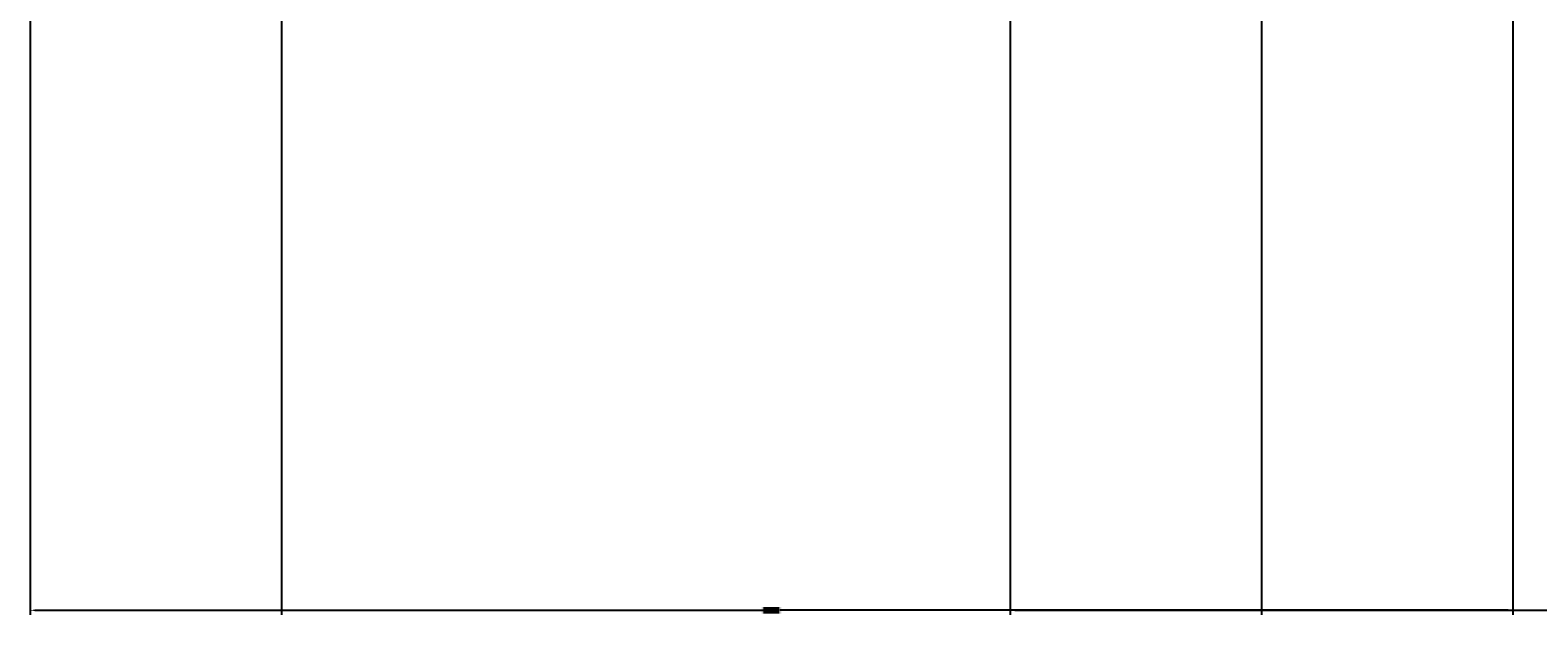
# Model space of a CAD drawing. Units: inches. Extents: x -128 to 854, y -395 to 398.
# Tile 3 of 61: x -76 to -16, y -382 to -359. Entities that reach past the tile are written whole.
import ezdxf

# ---------------------------------------------------------------- set-up
doc = ezdxf.new("R2010")
doc.units = ezdxf.units.IN
doc.header["$MEASUREMENT"] = 0
doc.layers.add('A-ANNO-DIMS', color=2, linetype='Continuous', lineweight=18)
doc.styles.get("Standard").update_dxf_attribs({"font": 'arial.ttf'})
doc.dimstyles.get("Standard").update_dxf_attribs({"dimtxt": 0.18, "dimasz": 0.18, "dimexe": 0.18, "dimexo": 0.0625, "dimgap": 0.09, "dimtad": 0, "dimtih": 1, "dimtoh": 1, "dimdec": 1, "dimzin": 0, "dimdsep": 46, "dimlunit": 4, "dimtxsty": 'Standard', "dimcen": 0.09, "dimclrd": 1, "dimclre": 2, "dimclrt": 6, "dimadec": 0, "dimazin": 0, "dimtfac": 1, "dimtdec": 1, "dimtofl": 0, "dimtmove": 0, "dimatfit": 3, "dimfxl": 1, "dimtfill": 2, "dimtfillclr": 3, "dimtolj": 1, "dimtzin": 0, "dimarcsym": 0})

# ---------------------------------------------------------------- blocks, each defined once
blk = doc.blocks.new('*D122')
at = {"layer": 'A-ANNO-DIMS', "color": 2, "lineweight": -2, "transparency": 16777216}
for p, q in [((-76.161, -358.082), (-76.161, -381.899)), ((-17.161, -358.082), (-17.161, -381.899))]:
    blk.add_line(p, q, dxfattribs=at)
at = {"layer": 'A-ANNO-DIMS', "color": 1, "lineweight": -2, "transparency": 16777216}
for p, q in [((-75.981, -381.719), (-47.064, -381.719)), ((-17.341, -381.719), (-46.258, -381.719))]:
    blk.add_line(p, q, dxfattribs=at)
at = {"layer": 'A-ANNO-DIMS', "color": 1, "transparency": 16777216}
for points in [[(-75.981, -381.689), (-75.981, -381.749), (-76.161, -381.719)], [(-17.341, -381.689), (-17.341, -381.749), (-17.161, -381.719)]]:
    blk.add_solid(points, dxfattribs=at)
at = {"layer": 'Defpoints', "color": 0, "transparency": 16777216}
for p in [(-76.161, -358.019), (-17.161, -358.019), (-17.161, -381.719)]:
    blk.add_point(p, dxfattribs=at)
at = {"layer": 'A-ANNO-DIMS', "color": 6, "transparency": 16777216, "insert": (-46.661, -381.719), "char_height": 0.18, "attachment_point": 5, "bg_fill": 1, "box_fill_scale": 1.25, "bg_fill_color": 3, "bg_fill_transparency": 0}
blk.add_mtext('\\A1;4\'-11"', dxfattribs=at)
blk = doc.blocks.new('*D123')
at = {"layer": 'A-ANNO-DIMS', "color": 2, "lineweight": -2, "transparency": 16777216}
for p, q in [((-17.161, -358.082), (-17.161, -381.899)), ((121.839, -358.082), (121.839, -381.899))]:
    blk.add_line(p, q, dxfattribs=at)
at = {"layer": 'A-ANNO-DIMS', "color": 1, "lineweight": -2, "transparency": 16777216}
for p, q in [((-16.981, -381.719), (51.948, -381.719)), ((121.659, -381.719), (52.73, -381.719))]:
    blk.add_line(p, q, dxfattribs=at)
at = {"layer": 'A-ANNO-DIMS', "color": 1, "transparency": 16777216}
for points in [[(-16.981, -381.689), (-16.981, -381.749), (-17.161, -381.719)], [(121.659, -381.689), (121.659, -381.749), (121.839, -381.719)]]:
    blk.add_solid(points, dxfattribs=at)
at = {"layer": 'Defpoints', "color": 0, "transparency": 16777216}
for p in [(-17.161, -358.019), (121.839, -358.019), (121.839, -381.719)]:
    blk.add_point(p, dxfattribs=at)
at = {"layer": 'A-ANNO-DIMS', "color": 6, "transparency": 16777216, "insert": (52.339, -381.719), "char_height": 0.18, "attachment_point": 5, "bg_fill": 1, "box_fill_scale": 1.25, "bg_fill_color": 3, "bg_fill_transparency": 0}
blk.add_mtext('\\A1;11\'-7"', dxfattribs=at)
blk = doc.blocks.new('*D125')
at = {"layer": 'A-ANNO-DIMS', "color": 2, "lineweight": -2, "transparency": 16777216}
for p, q in [((-37.161, -298.082), (-37.161, -381.899)), ((22.811, -298.082), (22.811, -381.899))]:
    blk.add_line(p, q, dxfattribs=at)
at = {"layer": 'A-ANNO-DIMS', "color": 1, "lineweight": -2, "transparency": 16777216}
for p, q in [((-36.981, -381.719), (-7.504, -381.719)), ((22.631, -381.719), (-6.846, -381.719))]:
    blk.add_line(p, q, dxfattribs=at)
at = {"layer": 'A-ANNO-DIMS', "color": 1, "transparency": 16777216}
for points in [[(-36.981, -381.689), (-36.981, -381.749), (-37.161, -381.719)], [(22.631, -381.689), (22.631, -381.749), (22.811, -381.719)]]:
    blk.add_solid(points, dxfattribs=at)
at = {"layer": 'Defpoints', "color": 0, "transparency": 16777216}
for p in [(-37.161, -298.019), (22.811, -298.019), (22.811, -381.719)]:
    blk.add_point(p, dxfattribs=at)
at = {"layer": 'A-ANNO-DIMS', "color": 6, "transparency": 16777216, "insert": (-7.175, -381.719), "char_height": 0.18, "attachment_point": 5, "bg_fill": 1, "box_fill_scale": 1.25, "bg_fill_color": 3, "bg_fill_transparency": 0}
blk.add_mtext('\\A1;5\'-0"', dxfattribs=at)
blk = doc.blocks.new('*D130')
at = {"layer": 'A-ANNO-DIMS', "color": 2, "lineweight": -2, "transparency": 16777216}
for p, q in [((-66.161, -322.082), (-66.161, -381.899)), ((-27.161, -322.082), (-27.161, -381.899))]:
    blk.add_line(p, q, dxfattribs=at)
at = {"layer": 'A-ANNO-DIMS', "color": 1, "lineweight": -2, "transparency": 16777216}
for p, q in [((-65.981, -381.719), (-46.99, -381.719)), ((-27.341, -381.719), (-46.332, -381.719))]:
    blk.add_line(p, q, dxfattribs=at)
at = {"layer": 'A-ANNO-DIMS', "color": 1, "transparency": 16777216}
for points in [[(-65.981, -381.689), (-65.981, -381.749), (-66.161, -381.719)], [(-27.341, -381.689), (-27.341, -381.749), (-27.161, -381.719)]]:
    blk.add_solid(points, dxfattribs=at)
at = {"layer": 'Defpoints', "color": 0, "transparency": 16777216}
for p in [(-66.161, -322.019), (-27.161, -322.019), (-27.161, -381.719)]:
    blk.add_point(p, dxfattribs=at)
at = {"layer": 'A-ANNO-DIMS', "color": 6, "transparency": 16777216, "insert": (-46.661, -381.719), "char_height": 0.18, "attachment_point": 5, "bg_fill": 1, "box_fill_scale": 1.25, "bg_fill_color": 3, "bg_fill_transparency": 0}
blk.add_mtext('\\A1;3\'-3"', dxfattribs=at)

msp = doc.modelspace()

# ---------------------------------------------------------------- dimensions: what is measured, and where the dimension line sits
at = {"layer": 'A-ANNO-DIMS'}
for base, p1, p2, picture, middle in [((22.811, -381.719), (-37.161, -298.019), (22.811, -298.019), '*D125', (-7.175, -381.719)), ((-27.161, -381.719), (-66.161, -322.019), (-27.161, -322.019), '*D130', (-46.661, -381.719)), ((-17.161, -381.719), (-76.161, -358.019), (-17.161, -358.019), '*D122', (-46.661, -381.719)), ((121.839, -381.719), (-17.161, -358.019), (121.839, -358.019), '*D123', (52.339, -381.719))]:
    dim = msp.add_linear_dim(base=base, p1=p1, p2=p2, dimstyle='Standard', override={"dimdec": 1, "dimlfac": 1, "dimrnd": 0, "dimzin": 1, "dimdsep": 46, "dimlunit": 4, "dimfrac": 2}, dxfattribs=at)
    dim.commit()
    dim.dimension.update_dxf_attribs({"geometry": picture, "text_midpoint": middle})

doc.saveas('drawing.dxf')
